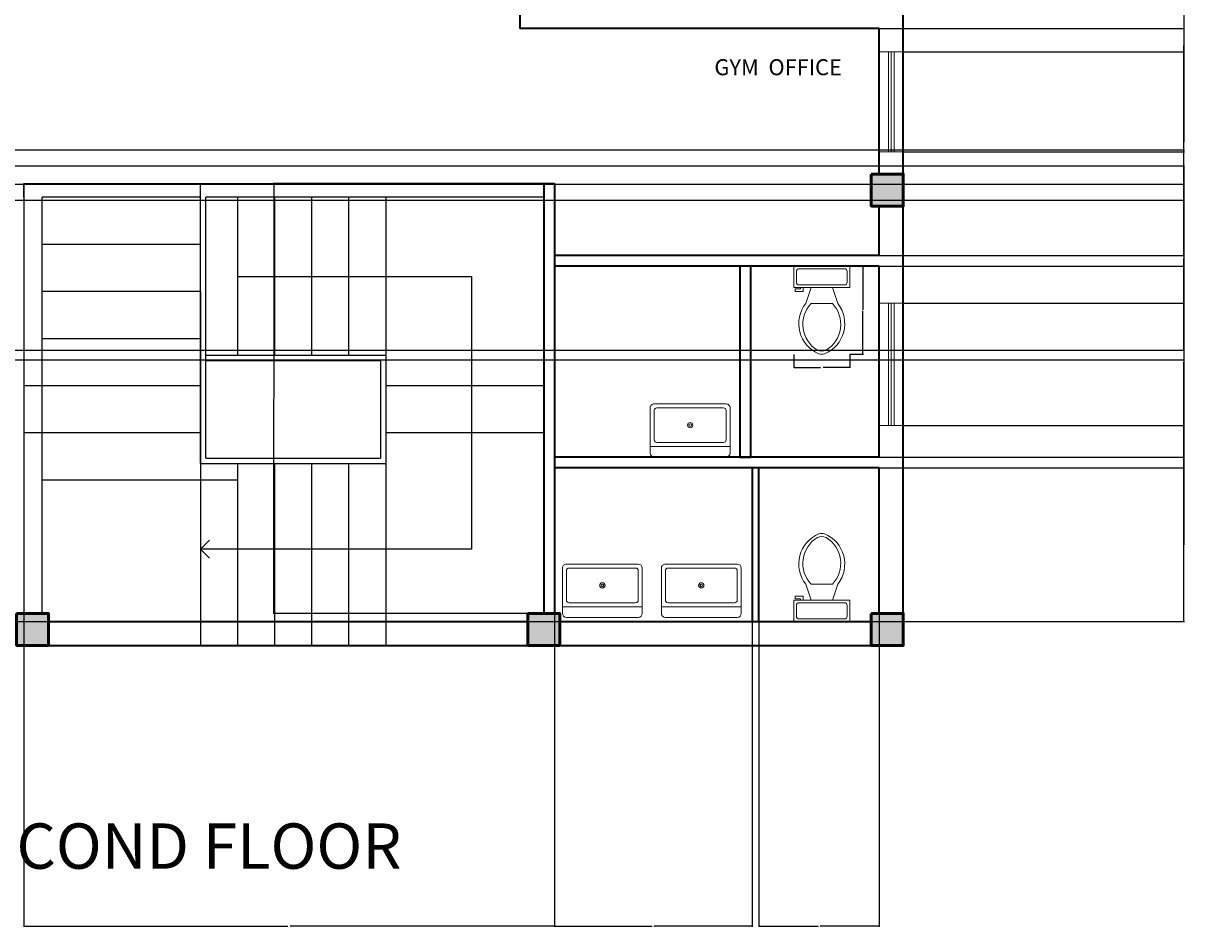
# Model space of a CAD drawing. Units: inches. Extents: x 369 to 4994, y 516 to 1297.
# Tile 8 of 9: x 2235 to 2672, y 516 to 855. Entities that reach past the tile are written whole.
import ezdxf

# ---------------------------------------------------------------- set-up
doc = ezdxf.new("R2010")
doc.units = ezdxf.units.IN
doc.header["$MEASUREMENT"] = 0
for name, color, linetype, lineweight in [('A-ANNO-DIMS', 2, 'Continuous', 18), ('A-ANNO-TEXT', 7, 'Continuous', 35), ('A-AREA-IDEN', 7, 'Continuous', 18), ('A-COLS', 7, 'Continuous', 50), ('A-FLOR-FIXT', 9, 'Continuous', 18), ('A-FLOR-STRS', 3, 'Continuous', 25), ('A-GLAZ', 4, 'Continuous', 18), ('A-WALL', 7, 'Continuous', 35)]:
    doc.layers.add(name, color=color, linetype=linetype, lineweight=lineweight)
doc.layers.add('A-COLS-PATT', color=18, linetype='Continuous', lineweight=13, true_color=0x000000)
doc.styles.get("Standard").update_dxf_attribs({"font": 'arial.ttf'})
doc.dimstyles.get("Standard").update_dxf_attribs({"dimtxt": 0.18, "dimasz": 0.18, "dimexe": 0.18, "dimexo": 0.0625, "dimgap": 0.09, "dimtad": 0, "dimtih": 1, "dimtoh": 1, "dimdec": 4, "dimzin": 0, "dimdsep": 46, "dimtxsty": 'Standard', "dimcen": 0.09, "dimadec": 0, "dimazin": 0, "dimtfac": 1, "dimtdec": 4, "dimtofl": 0, "dimtmove": 0, "dimatfit": 3, "dimfxl": 1, "dimtolj": 1, "dimtzin": 0, "dimarcsym": 0})

# ---------------------------------------------------------------- blocks, each defined once
blk = doc.blocks.new('Toilet - top')
for p, q in [((9.5, -6), (9.5, -2)), ((-10, -8.5), (-8, -8.5)), ((-10, -9.5), (-10, -8.5)), ((-8, -8.5), (-8, -8)), ((-7, -8), (-7, -9.5)), ((-4, -8), (-6, -14)), ((4, -8), (6, -14)), ((-7, -9.5), (-10, -9.5)), ((4, -14), (-4, -14))]:
    blk.add_line(p, q)
blk.add_lwpolyline([(10.5, -8), (10.5, 0), (-10.5, 0), (-10.5, -8)], close=True)
for points in [[(-9.5, -2), (-9.5, -6)], [(8.5, -1), (-8.5, -1)], [(-8.5, -7), (8.5, -7)]]:
    blk.add_lwpolyline(points)
for centre, radius, start, end in [((-8.62, -1.88), 0.884, 81.8699, 188.1301), ((8.62, -1.88), 0.884, 351.8699, 98.1301), ((-8.62, -6.12), 0.884, 171.8699, 278.1301), ((8.62, -6.12), 0.884, 261.8699, 8.1301), ((3.52, -21.58), 12.17, 141.4691, 247.9714), ((4.2, -21.82), 11.33, 136.3677, 238.9468), ((-3.52, -21.58), 12.17, 292.0284, 38.5307), ((-4.2, -21.82), 11.33, 301.053, 43.6321), ((0, -27.88), 4, 245.7318, 294.2682), ((0, -29), 4, 254.8605, 285.1395)]:
    blk.add_arc(centre, radius, start, end)
blk = doc.blocks.new('Sink-single - 30 in top')
blk.add_line((-15, -3.999996), (15, -3.999996))
for points in [[(-13.5, 0), (13.5, 0)], [(-15, -18.499996), (-15, -1.5)], [(15, -1.5), (15, -18.499996)], [(-13.5, -17.499996), (-13.5, -6.499996)], [(-12.5, -5.499996), (12.5, -5.499996)], [(13.5, -6.499996), (13.5, -17.499996)], [(13.5, -19.999996), (-13.5, -19.999996)], [(12.5, -18.499996), (-12.5, -18.499996)]]:
    blk.add_lwpolyline(points)
for radius in [1, 0.5]:
    blk.add_circle((0, -11.999996), radius)
for centre, radius, start, end in [((-13.5, -1.5), 1.5, 90, 180), ((13.5, -1.5), 1.5, 0, 90), ((-12.5, -6.499996), 1, 90, 180), ((12.5, -6.499996), 1, 0, 90), ((-13.5, -18.499996), 1.5, 180, 270), ((-12.5, -17.499996), 1, 180, 270), ((12.5, -17.499996), 1, 270, 0), ((13.5, -18.499996), 1.5, 270, 0)]:
    blk.add_arc(centre, radius, start, end)
blk = doc.blocks.new('*D25')
at = {"layer": 'A-ANNO-DIMS', "color": 0, "lineweight": -2, "transparency": 16777216}
for p, q in [((2545.87, 764.15), (2550.95, 764.15)), ((2550.77, 763.97), (2550.77, 747.81)), ((2550.77, 731.28), (2550.77, 747.44)), ((2545.87, 731.1), (2550.95, 731.1))]:
    blk.add_line(p, q, dxfattribs=at)
at = {"layer": 'A-ANNO-DIMS', "color": 0, "transparency": 16777216}
for points in [[(2550.74, 763.97), (2550.8, 763.97), (2550.77, 764.15)], [(2550.74, 731.28), (2550.8, 731.28), (2550.77, 731.1)]]:
    blk.add_solid(points, dxfattribs=at)
at = {"layer": 'Defpoints', "color": 0, "transparency": 16777216}
for p in [(2545.81, 764.15), (2550.77, 764.15), (2545.81, 731.1)]:
    blk.add_point(p, dxfattribs=at)
at = {"layer": 'A-ANNO-DIMS', "color": 0, "transparency": 16777216, "insert": (2550.77, 747.63), "char_height": 0.18, "attachment_point": 5}
blk.add_mtext('\\A1;WC 33 TYP.', dxfattribs=at)
blk = doc.blocks.new('*D26')
at = {"layer": 'A-ANNO-DIMS', "color": 0, "lineweight": -2, "transparency": 16777216}
for p, q in [((2524.81, 731.04), (2524.81, 725.97)), ((2545.81, 731.04), (2545.81, 725.97)), ((2524.99, 726.15), (2534.78, 726.15)), ((2545.63, 726.15), (2535.84, 726.15))]:
    blk.add_line(p, q, dxfattribs=at)
at = {"layer": 'A-ANNO-DIMS', "color": 0, "transparency": 16777216}
for points in [[(2524.99, 726.18), (2524.99, 726.12), (2524.81, 726.15)], [(2545.63, 726.18), (2545.63, 726.12), (2545.81, 726.15)]]:
    blk.add_solid(points, dxfattribs=at)
at = {"layer": 'Defpoints', "color": 0, "transparency": 16777216}
for p in [(2524.81, 731.1), (2545.81, 731.1), (2545.81, 726.15)]:
    blk.add_point(p, dxfattribs=at)
at = {"layer": 'A-ANNO-DIMS', "color": 0, "transparency": 16777216, "insert": (2535.31, 726.15), "char_height": 0.18, "attachment_point": 5}
blk.add_mtext('\\A1;21 TYP.', dxfattribs=at)
blk = doc.blocks.new('*D47')
at = {"layer": 'A-ANNO-DIMS', "color": 0, "lineweight": -2, "transparency": 16777216}
for p, q in [((1038.32, 879.79), (2671.51, 879.79)), ((2671.33, 879.61), (2671.33, 837.52)), ((2671.33, 795.07), (2671.33, 837.16)), ((1035.32, 794.89), (2671.51, 794.89))]:
    blk.add_line(p, q, dxfattribs=at)
at = {"layer": 'A-ANNO-DIMS', "color": 0, "transparency": 16777216}
for points in [[(2671.3, 879.61), (2671.36, 879.61), (2671.33, 879.79)], [(2671.3, 795.07), (2671.36, 795.07), (2671.33, 794.89)]]:
    blk.add_solid(points, dxfattribs=at)
at = {"layer": 'Defpoints', "color": 0, "transparency": 16777216}
for p in [(1038.26, 879.79), (2671.33, 879.79), (1035.26, 794.89)]:
    blk.add_point(p, dxfattribs=at)
at = {"layer": 'A-ANNO-DIMS', "color": 0, "transparency": 16777216, "insert": (2671.33, 837.34), "char_height": 0.18, "attachment_point": 5}
blk.add_mtext('\\A1;84.9', dxfattribs=at)
blk = doc.blocks.new('*D52')
at = {"layer": 'A-ANNO-DIMS', "color": 0, "lineweight": -2, "transparency": 16777216}
for p, q in [((942.32, 788.89), (2671.51, 788.89)), ((2671.33, 788.71), (2671.33, 710.02)), ((2671.33, 630.97), (2671.33, 709.66)), ((1035.32, 630.79), (2671.51, 630.79))]:
    blk.add_line(p, q, dxfattribs=at)
at = {"layer": 'A-ANNO-DIMS', "color": 0, "transparency": 16777216}
for points in [[(2671.3, 788.71), (2671.36, 788.71), (2671.33, 788.89)], [(2671.3, 630.97), (2671.36, 630.97), (2671.33, 630.79)]]:
    blk.add_solid(points, dxfattribs=at)
at = {"layer": 'Defpoints', "color": 0, "transparency": 16777216}
for p in [(942.26, 788.89), (2671.33, 788.89), (1035.26, 630.79)]:
    blk.add_point(p, dxfattribs=at)
at = {"layer": 'A-ANNO-DIMS', "color": 0, "transparency": 16777216, "insert": (2671.33, 709.84), "char_height": 0.18, "attachment_point": 5}
blk.add_mtext('\\A1;158.1', dxfattribs=at)
blk = doc.blocks.new('*D80')
at = {"layer": 'A-ANNO-DIMS', "color": 0, "lineweight": -2, "transparency": 16777216}
for p, q in [((1772.44, 886.6), (2671.51, 886.6)), ((2671.33, 886.42), (2671.33, 847.38)), ((2671.33, 807.97), (2671.33, 847.01)), ((1772.44, 807.79), (2671.51, 807.79))]:
    blk.add_line(p, q, dxfattribs=at)
at = {"layer": 'A-ANNO-DIMS', "color": 0, "transparency": 16777216}
for points in [[(2671.3, 886.42), (2671.36, 886.42), (2671.33, 886.6)], [(2671.3, 807.97), (2671.36, 807.97), (2671.33, 807.79)]]:
    blk.add_solid(points, dxfattribs=at)
at = {"layer": 'Defpoints', "color": 0, "transparency": 16777216}
for p in [(1772.37, 886.6), (2671.33, 886.6), (1772.37, 807.79)]:
    blk.add_point(p, dxfattribs=at)
at = {"layer": 'A-ANNO-DIMS', "color": 0, "transparency": 16777216, "insert": (2671.33, 847.19), "char_height": 0.18, "attachment_point": 5}
blk.add_mtext('\\A1;78.81', dxfattribs=at)
blk = doc.blocks.new('*D85')
at = {"layer": 'A-ANNO-DIMS', "color": 0, "lineweight": -2, "transparency": 16777216}
for p, q in [((1772.44, 801.79), (2671.51, 801.79)), ((2671.33, 801.61), (2671.33, 767.36)), ((2671.33, 732.75), (2671.33, 767)), ((1772.44, 732.57), (2671.51, 732.57))]:
    blk.add_line(p, q, dxfattribs=at)
at = {"layer": 'A-ANNO-DIMS', "color": 0, "transparency": 16777216}
for points in [[(2671.3, 801.61), (2671.36, 801.61), (2671.33, 801.79)], [(2671.3, 732.75), (2671.36, 732.75), (2671.33, 732.57)]]:
    blk.add_solid(points, dxfattribs=at)
at = {"layer": 'Defpoints', "color": 0, "transparency": 16777216}
for p in [(1772.37, 801.79), (2671.33, 801.79), (1772.37, 732.57)]:
    blk.add_point(p, dxfattribs=at)
at = {"layer": 'A-ANNO-DIMS', "color": 0, "transparency": 16777216, "insert": (2671.33, 767.18), "char_height": 0.18, "attachment_point": 5}
blk.add_mtext('\\A1;69.22', dxfattribs=at)
blk = doc.blocks.new('*D86')
at = {"layer": 'A-ANNO-DIMS', "color": 0, "lineweight": -2, "transparency": 16777216}
for p, q in [((1772.44, 728.97), (2671.51, 728.97)), ((2671.33, 728.79), (2671.33, 680.06)), ((2671.33, 630.97), (2671.33, 679.7)), ((1769.44, 630.79), (2671.51, 630.79))]:
    blk.add_line(p, q, dxfattribs=at)
at = {"layer": 'A-ANNO-DIMS', "color": 0, "transparency": 16777216}
for points in [[(2671.3, 728.79), (2671.36, 728.79), (2671.33, 728.97)], [(2671.3, 630.97), (2671.36, 630.97), (2671.33, 630.79)]]:
    blk.add_solid(points, dxfattribs=at)
at = {"layer": 'Defpoints', "color": 0, "transparency": 16777216}
for p in [(1772.37, 728.97), (2671.33, 728.97), (1769.37, 630.79)]:
    blk.add_point(p, dxfattribs=at)
at = {"layer": 'A-ANNO-DIMS', "color": 0, "transparency": 16777216, "insert": (2671.33, 679.88), "char_height": 0.18, "attachment_point": 5}
blk.add_mtext('\\A1;98.18', dxfattribs=at)
blk = doc.blocks.new('*D105')
at = {"layer": 'A-ANNO-DIMS', "color": 0, "lineweight": -2, "transparency": 16777216}
for p, q in [((2556.99, 853.34), (2671.51, 853.34)), ((2671.33, 853.16), (2671.33, 810.93)), ((2671.33, 768.33), (2671.33, 810.56)), ((2556.99, 768.15), (2671.51, 768.15))]:
    blk.add_line(p, q, dxfattribs=at)
at = {"layer": 'A-ANNO-DIMS', "color": 0, "transparency": 16777216}
for points in [[(2671.3, 853.16), (2671.36, 853.16), (2671.33, 853.34)], [(2671.3, 768.33), (2671.36, 768.33), (2671.33, 768.15)]]:
    blk.add_solid(points, dxfattribs=at)
at = {"layer": 'Defpoints', "color": 0, "transparency": 16777216}
for p in [(2556.93, 853.34), (2671.33, 853.34), (2556.93, 768.15)]:
    blk.add_point(p, dxfattribs=at)
at = {"layer": 'A-ANNO-DIMS', "color": 0, "transparency": 16777216, "insert": (2671.33, 810.75), "char_height": 0.18, "attachment_point": 5}
blk.add_mtext('\\A1;85.19', dxfattribs=at)
blk = doc.blocks.new('*D106')
at = {"layer": 'A-ANNO-DIMS', "color": 0, "lineweight": -2, "transparency": 16777216}
for p, q in [((2556.99, 764.15), (2671.51, 764.15)), ((2671.33, 763.97), (2671.33, 728.5)), ((2671.33, 692.66), (2671.33, 728.13)), ((2556.99, 692.48), (2671.51, 692.48))]:
    blk.add_line(p, q, dxfattribs=at)
at = {"layer": 'A-ANNO-DIMS', "color": 0, "transparency": 16777216}
for points in [[(2671.3, 763.97), (2671.36, 763.97), (2671.33, 764.15)], [(2671.3, 692.66), (2671.36, 692.66), (2671.33, 692.48)]]:
    blk.add_solid(points, dxfattribs=at)
at = {"layer": 'Defpoints', "color": 0, "transparency": 16777216}
for p in [(2556.93, 764.15), (2671.33, 764.15), (2556.93, 692.48)]:
    blk.add_point(p, dxfattribs=at)
at = {"layer": 'A-ANNO-DIMS', "color": 0, "transparency": 16777216, "insert": (2671.33, 728.32), "char_height": 0.18, "attachment_point": 5}
blk.add_mtext('\\A1;71.67', dxfattribs=at)
blk = doc.blocks.new('*D107')
at = {"layer": 'A-ANNO-DIMS', "color": 0, "lineweight": -2, "transparency": 16777216}
for p, q in [((2556.99, 688.48), (2671.51, 688.48)), ((2671.33, 688.3), (2671.33, 659.82)), ((2671.33, 630.97), (2671.33, 659.45)), ((2553.99, 630.79), (2671.51, 630.79))]:
    blk.add_line(p, q, dxfattribs=at)
at = {"layer": 'A-ANNO-DIMS', "color": 0, "transparency": 16777216}
for points in [[(2671.3, 688.3), (2671.36, 688.3), (2671.33, 688.48)], [(2671.3, 630.97), (2671.36, 630.97), (2671.33, 630.79)]]:
    blk.add_solid(points, dxfattribs=at)
at = {"layer": 'Defpoints', "color": 0, "transparency": 16777216}
for p in [(2556.93, 688.48), (2671.33, 688.48), (2553.93, 630.79)]:
    blk.add_point(p, dxfattribs=at)
at = {"layer": 'A-ANNO-DIMS', "color": 0, "transparency": 16777216, "insert": (2671.33, 659.64), "char_height": 0.18, "attachment_point": 5}
blk.add_mtext('\\A1;57.69', dxfattribs=at)
blk = doc.blocks.new('*D109')
at = {"layer": 'A-ANNO-DIMS', "color": 0, "lineweight": -2, "transparency": 16777216}
for p, q in [((2235.65, 795.12), (2235.65, 516.21)), ((2434.93, 795.12), (2434.93, 516.21)), ((2235.83, 516.39), (2334.83, 516.39)), ((2434.75, 516.39), (2335.74, 516.39))]:
    blk.add_line(p, q, dxfattribs=at)
at = {"layer": 'A-ANNO-DIMS', "color": 0, "transparency": 16777216}
for points in [[(2235.83, 516.42), (2235.83, 516.36), (2235.65, 516.39)], [(2434.75, 516.42), (2434.75, 516.36), (2434.93, 516.39)]]:
    blk.add_solid(points, dxfattribs=at)
at = {"layer": 'Defpoints', "color": 0, "transparency": 16777216}
for p in [(2235.65, 795.19), (2434.93, 795.19), (2434.93, 516.39)]:
    blk.add_point(p, dxfattribs=at)
at = {"layer": 'A-ANNO-DIMS', "color": 0, "transparency": 16777216, "insert": (2335.29, 516.39), "char_height": 0.18, "attachment_point": 5}
blk.add_mtext('\\A1;199.27', dxfattribs=at)
blk = doc.blocks.new('*D110')
at = {"layer": 'A-ANNO-DIMS', "color": 0, "lineweight": -2, "transparency": 16777216}
for p, q in [((2434.93, 688.42), (2434.93, 516.21)), ((2509.12, 688.42), (2509.12, 516.21)), ((2435.11, 516.39), (2471.63, 516.39)), ((2508.94, 516.39), (2472.42, 516.39))]:
    blk.add_line(p, q, dxfattribs=at)
at = {"layer": 'A-ANNO-DIMS', "color": 0, "transparency": 16777216}
for points in [[(2435.11, 516.42), (2435.11, 516.36), (2434.93, 516.39)], [(2508.94, 516.42), (2508.94, 516.36), (2509.12, 516.39)]]:
    blk.add_solid(points, dxfattribs=at)
at = {"layer": 'Defpoints', "color": 0, "transparency": 16777216}
for p in [(2434.93, 688.48), (2509.12, 688.48), (2509.12, 516.39)]:
    blk.add_point(p, dxfattribs=at)
at = {"layer": 'A-ANNO-DIMS', "color": 0, "transparency": 16777216, "insert": (2472.02, 516.39), "char_height": 0.18, "attachment_point": 5}
blk.add_mtext('\\A1;74.19', dxfattribs=at)
blk = doc.blocks.new('*D111')
at = {"layer": 'A-ANNO-DIMS', "color": 0, "lineweight": -2, "transparency": 16777216}
for p, q in [((2511.66, 688.42), (2511.66, 516.21)), ((2556.93, 688.42), (2556.93, 516.21)), ((2511.84, 516.39), (2533.9, 516.39)), ((2556.75, 516.39), (2534.69, 516.39))]:
    blk.add_line(p, q, dxfattribs=at)
at = {"layer": 'A-ANNO-DIMS', "color": 0, "transparency": 16777216}
for points in [[(2511.84, 516.42), (2511.84, 516.36), (2511.66, 516.39)], [(2556.75, 516.42), (2556.75, 516.36), (2556.93, 516.39)]]:
    blk.add_solid(points, dxfattribs=at)
at = {"layer": 'Defpoints', "color": 0, "transparency": 16777216}
for p in [(2511.66, 688.48), (2556.93, 688.48), (2556.93, 516.39)]:
    blk.add_point(p, dxfattribs=at)
at = {"layer": 'A-ANNO-DIMS', "color": 0, "transparency": 16777216, "insert": (2534.29, 516.39), "char_height": 0.18, "attachment_point": 5}
blk.add_mtext('\\A1;45.27', dxfattribs=at)
blk = doc.blocks.new('*D118')
at = {"layer": 'A-ANNO-DIMS', "color": 0, "lineweight": -2, "transparency": 16777216}
for p, q in [((2565.99, 844.57), (2671.51, 844.57)), ((2671.33, 844.39), (2671.33, 826.03)), ((2671.33, 807.3), (2671.33, 825.66)), ((2565.99, 807.12), (2671.51, 807.12))]:
    blk.add_line(p, q, dxfattribs=at)
at = {"layer": 'A-ANNO-DIMS', "color": 0, "transparency": 16777216}
for points in [[(2671.3, 844.39), (2671.36, 844.39), (2671.33, 844.57)], [(2671.3, 807.3), (2671.36, 807.3), (2671.33, 807.12)]]:
    blk.add_solid(points, dxfattribs=at)
at = {"layer": 'Defpoints', "color": 0, "transparency": 16777216}
for p in [(2565.93, 844.57), (2565.93, 807.12), (2671.33, 807.12)]:
    blk.add_point(p, dxfattribs=at)
at = {"layer": 'A-ANNO-DIMS', "color": 0, "transparency": 16777216, "insert": (2671.33, 825.84), "char_height": 0.18, "attachment_point": 5}
blk.add_mtext('\\A1;37.45', dxfattribs=at)
blk = doc.blocks.new('*D119')
at = {"layer": 'A-ANNO-DIMS', "color": 0, "lineweight": -2, "transparency": 16777216}
for p, q in [((2565.99, 750.32), (2671.51, 750.32)), ((2671.33, 750.14), (2671.33, 727.55)), ((2671.33, 704.59), (2671.33, 727.18)), ((2565.99, 704.41), (2671.51, 704.41))]:
    blk.add_line(p, q, dxfattribs=at)
at = {"layer": 'A-ANNO-DIMS', "color": 0, "transparency": 16777216}
for points in [[(2671.3, 750.14), (2671.36, 750.14), (2671.33, 750.32)], [(2671.3, 704.59), (2671.36, 704.59), (2671.33, 704.41)]]:
    blk.add_solid(points, dxfattribs=at)
at = {"layer": 'Defpoints', "color": 0, "transparency": 16777216}
for p in [(2565.93, 750.32), (2565.93, 704.41), (2671.33, 704.41)]:
    blk.add_point(p, dxfattribs=at)
at = {"layer": 'A-ANNO-DIMS', "color": 0, "transparency": 16777216, "insert": (2671.33, 727.36), "char_height": 0.18, "attachment_point": 5}
blk.add_mtext('\\A1;45.91', dxfattribs=at)
blk = doc.blocks.new('*D121')
at = {"layer": 'A-ANNO-DIMS', "color": 0, "lineweight": -2, "transparency": 16777216}
for p, q in [((2434.86, 795.19), (2329.35, 795.19)), ((2329.53, 795.01), (2329.53, 714.67)), ((2329.53, 633.97), (2329.53, 714.31)), ((2434.86, 633.79), (2329.35, 633.79))]:
    blk.add_line(p, q, dxfattribs=at)
at = {"layer": 'A-ANNO-DIMS', "color": 0, "transparency": 16777216}
for points in [[(2329.5, 795.01), (2329.56, 795.01), (2329.53, 795.19)], [(2329.5, 633.97), (2329.56, 633.97), (2329.53, 633.79)]]:
    blk.add_solid(points, dxfattribs=at)
at = {"layer": 'Defpoints', "color": 0, "transparency": 16777216}
for p in [(2329.53, 795.19), (2434.93, 795.19), (2434.93, 633.79)]:
    blk.add_point(p, dxfattribs=at)
at = {"layer": 'A-ANNO-DIMS', "color": 0, "transparency": 16777216, "insert": (2329.53, 714.49), "char_height": 0.18, "attachment_point": 5}
blk.add_mtext('\\A1;161.4', dxfattribs=at)

msp = doc.modelspace()

# ---------------------------------------------------------------- hatches: boundary and pattern name
at = {"layer": 'A-COLS-PATT'}
h = msp.add_hatch(color=256, dxfattribs=at)
h.dxf.hatch_style = 1
h.paths.add_polyline_path([(540.2581, 633.7894), (528.2581, 633.7894), (528.2581, 621.7894), (540.2581, 621.7894)])
h.paths.add_polyline_path([(726.2581, 633.7894), (714.2581, 633.7894), (714.2581, 621.7894), (726.2581, 621.7894)])
h.paths.add_polyline_path([(918.2581, 633.7894), (906.2581, 633.7894), (906.2581, 621.7894), (918.2581, 621.7894)])
h.paths.add_polyline_path([(1047.2581, 633.7894), (1035.2581, 633.7894), (1035.2581, 621.7894), (1047.2581, 621.7894)])
h.paths.add_polyline_path([(1047.2581, 798.6977), (1035.2581, 798.6977), (1035.2581, 786.6977), (1047.2581, 786.6977)])
h.paths.add_polyline_path([(918.2581, 795.7894), (906.2581, 795.7894), (906.2581, 783.7894), (918.2581, 783.7894)])
h.paths.add_polyline_path([(726.2581, 795.7894), (714.2581, 795.7894), (714.2581, 783.7894), (726.2581, 783.7894)])
h.paths.add_polyline_path([(1047.2581, 1038.7894), (1035.2581, 1038.7894), (1035.2581, 1026.7894), (1047.2581, 1026.7894)])
h.paths.add_polyline_path([(855.044, 1038.7894), (843.044, 1038.7894), (843.044, 1026.7894), (855.044, 1026.7894)])
h.paths.add_polyline_path([(728.5536, 1038.7894), (716.5536, 1038.7894), (716.5536, 1026.7894), (728.5536, 1026.7894)])
h.paths.add_polyline_path([(543.2581, 1038.7894), (531.2581, 1038.7894), (531.2581, 1026.7894), (543.2581, 1026.7894)])
h.paths.add_polyline_path([(543.2581, 792.9013), (531.2581, 792.9013), (531.2581, 780.9013), (543.2581, 780.9013), (543.2581, 783.7894)])
h.paths.add_polyline_path([(1274.3738, 633.7894), (1262.3738, 633.7894), (1262.3738, 621.7894), (1274.3738, 621.7894)])
h.paths.add_polyline_path([(1460.3738, 633.7894), (1448.3738, 633.7894), (1448.3738, 621.7894), (1460.3738, 621.7894)])
h.paths.add_polyline_path([(1652.3738, 633.7894), (1640.3738, 633.7894), (1640.3738, 621.7894), (1652.3738, 621.7894)])
h.paths.add_polyline_path([(1781.3738, 633.7894), (1769.3738, 633.7894), (1769.3738, 621.7894), (1781.3738, 621.7894)])
h.paths.add_polyline_path([(1781.3738, 1038.7894), (1769.3738, 1038.7894), (1769.3738, 1026.7894), (1781.3738, 1026.7894)])
h.paths.add_polyline_path([(1625.484, 1038.7894), (1613.484, 1038.7894), (1613.484, 1026.7894), (1615.6962, 1026.7894), (1625.484, 1026.7894)])
h.paths.add_polyline_path([(1462.6692, 1038.7894), (1450.6692, 1038.7894), (1450.6692, 1026.7894), (1462.6692, 1026.7894)])
h.paths.add_polyline_path([(1277.3738, 1038.7894), (1265.3738, 1038.7894), (1265.3738, 1026.7894), (1277.3738, 1026.7894)])
h.paths.add_polyline_path([(1460.3738, 807.7894), (1448.3738, 807.7894), (1448.3738, 795.7894), (1460.3738, 795.7894)])
h.paths.add_polyline_path([(1652.3738, 807.7894), (1640.3738, 807.7894), (1640.3738, 795.7894), (1652.3738, 795.7894)])
h.paths.add_polyline_path([(2244.9265, 633.7894), (2232.9265, 633.7894), (2232.9265, 621.7894), (2244.9265, 621.7894)])
h.paths.add_polyline_path([(2058.9265, 633.7894), (2046.9265, 633.7894), (2046.9265, 621.7894), (2058.9265, 621.7894)])
h.paths.add_polyline_path([(2436.9265, 633.7894), (2424.9265, 633.7894), (2424.9265, 621.7894), (2436.9265, 621.7894)])
h.paths.add_polyline_path([(2565.9265, 633.7894), (2553.9265, 633.7894), (2553.9265, 621.7894), (2565.9265, 621.7894)])
h.paths.add_polyline_path([(2565.9265, 798.6977), (2553.9265, 798.6977), (2553.9265, 786.6977), (2565.9265, 786.6977)])
h.paths.add_polyline_path([(2565.9265, 1038.7894), (2553.9265, 1038.7894), (2553.9265, 1026.7894), (2565.9265, 1026.7894)])
h.paths.add_polyline_path([(2436.9265, 1038.7894), (2424.9265, 1038.7894), (2424.9265, 1026.7894), (2436.9265, 1026.7894)])
h.paths.add_polyline_path([(2247.222, 1038.7894), (2235.222, 1038.7894), (2235.222, 1026.7894), (2247.222, 1026.7894)])
h.paths.add_polyline_path([(2061.9265, 1038.7894), (2049.9265, 1038.7894), (2049.9265, 1026.7894), (2061.9265, 1026.7894)])

# ---------------------------------------------------------------- linework, layer by layer
at = {"layer": 'A-COLS'}
for points in [[(2553.9265, 798.6977), (2565.9265, 798.6977), (2565.9265, 786.6977), (2553.9265, 786.6977)], [(2232.9265, 633.7894), (2244.9265, 633.7894), (2244.9265, 621.7894), (2232.9265, 621.7894)], [(2424.9265, 633.7894), (2436.9265, 633.7894), (2436.9265, 621.7894), (2424.9265, 621.7894)], [(2553.9265, 633.7894), (2565.9265, 633.7894), (2565.9265, 621.7894), (2553.9265, 621.7894)]]:
    msp.add_lwpolyline(points, close=True, dxfattribs=at)
at = {"layer": 'A-FLOR-STRS'}
for p, q in [((2235.6525, 795.1866), (2235.6525, 633.7894)), ((2301.9505, 690.1533), (2301.9505, 795.1866)), ((2430.9265, 795.1866), (2434.9265, 795.1866)), ((2242.5867, 633.7894), (2242.5867, 790.0048)), ((2303.9505, 692.1533), (2303.9505, 790.0048)), ((2315.873, 790.0048), (2315.873, 730.6409)), ((2329.7954, 790.0048), (2329.7954, 730.6409)), ((2343.7178, 790.0048), (2343.7178, 730.6409)), ((2357.6402, 790.0048), (2357.6402, 730.6409)), ((2371.5626, 790.0048), (2371.5626, 621.7894)), ((2371.5626, 790.0048), (2371.5626, 621.7894)), ((2315.873, 760.3228), (2403.7562, 760.3228)), ((2403.7562, 760.3228), (2403.7562, 657.9608)), ((2301.9505, 754.6236), (2301.9505, 621.7894)), ((2369.5626, 728.6409), (2369.5626, 692.1533)), ((2371.5626, 730.6409), (2371.5626, 690.1533)), ((2301.9505, 690.1533), (2371.5626, 690.1533)), ((2303.9505, 692.1533), (2369.5626, 692.1533)), ((2315.873, 690.1533), (2315.873, 621.7894)), ((2329.7954, 690.1533), (2329.7954, 621.7894)), ((2343.7178, 690.1533), (2343.7178, 621.7894)), ((2357.6402, 690.1533), (2357.6402, 621.7894)), ((2301.9505, 657.9608), (2305.3296, 661.3398)), ((2403.7562, 657.9608), (2301.9505, 657.9608)), ((2301.9505, 657.9608), (2305.3296, 654.5817)), ((2235.6525, 633.7894), (2242.5867, 633.7894)), ((2303.9505, 630.7894), (2369.5626, 630.7894))]:
    msp.add_line(p, q, dxfattribs=at)
for points in [[(2235.6525, 790.0048), (2235.6525, 795.1866), (2430.9265, 795.1866)], [(2301.9505, 790.0048), (2242.5867, 790.0048)], [(2430.9265, 790.0048), (2303.9505, 790.0048)], [(2301.9505, 772.3142), (2242.5867, 772.3142)], [(2301.9505, 754.6236), (2242.5867, 754.6236)], [(2301.9505, 736.933), (2242.5867, 736.933)], [(2371.5626, 730.6409), (2303.9505, 730.6409)], [(2369.5626, 728.6409), (2303.9505, 728.6409)], [(2301.9505, 719.2424), (2235.6525, 719.2424)], [(2430.9265, 719.2424), (2371.5626, 719.2424)], [(2301.9505, 701.5518), (2235.6525, 701.5518)], [(2430.9265, 701.5518), (2371.5626, 701.5518)], [(2315.873, 683.8612), (2242.5867, 683.8612)], [(2301.9505, 630.7894), (2244.9265, 630.7894)]]:
    msp.add_lwpolyline(points, dxfattribs=at)
at = {"layer": 'A-GLAZ'}
for p, q in [((2560.3504, 807.1195), (2560.3504, 844.5673)), ((2561.4265, 807.1195), (2561.4265, 844.5673)), ((2562.5026, 807.1195), (2562.5026, 844.5673)), ((2560.3504, 704.4093), (2560.3504, 750.3191)), ((2561.4265, 704.4093), (2561.4265, 750.3191)), ((2562.5026, 704.4093), (2562.5026, 750.3191))]:
    msp.add_line(p, q, dxfattribs=at)
for points in [[(2556.9265, 807.1195), (2565.9265, 807.1195), (2565.9265, 844.5673), (2556.9265, 844.5673)], [(2556.9265, 704.4093), (2565.9265, 704.4093), (2565.9265, 750.3191), (2556.9265, 750.3191)]]:
    msp.add_lwpolyline(points, close=True, dxfattribs=at)
at = {"layer": 'A-WALL'}
for p, q in [((2565.9265, 621.7894), (2565.9265, 1029.7894)), ((2421.9265, 908.8078), (2421.9265, 853.3402)), ((2430.9265, 853.3402), (2421.9265, 853.3402)), ((2556.9265, 853.3402), (2430.9265, 853.3402)), ((2556.9265, 798.6977), (2556.9265, 853.3402)), ((2556.9265, 798.6977), (2556.9265, 853.3402)), ((2430.9265, 795.1866), (2430.9265, 768.15)), ((2430.9265, 795.1866), (2430.9265, 633.7894)), ((2434.9265, 795.1866), (2434.9265, 688.4833)), ((2556.9265, 771.7894), (2556.9265, 786.6977)), ((2556.9265, 768.15), (2556.9265, 786.6977)), ((2556.9265, 768.15), (2434.9265, 768.15)), ((2434.9265, 768.15), (2434.9265, 692.4833)), ((2556.9265, 764.15), (2434.9265, 764.15)), ((2556.9265, 692.4833), (2556.9265, 764.15)), ((2430.9265, 692.4833), (2430.9265, 633.7894)), ((2556.9265, 692.4833), (2434.9265, 692.4833)), ((2556.9265, 688.4833), (2434.9265, 688.4833)), ((2434.9265, 688.4833), (2434.9265, 633.7894)), ((2556.9265, 633.7894), (2556.9265, 688.4833)), ((2244.9265, 630.7894), (2424.9265, 630.7894)), ((2436.9265, 630.7894), (2466.1551, 630.7894)), ((2436.9265, 630.7894), (2553.9265, 630.7894)), ((2244.9265, 621.7894), (2436.9265, 621.7894)), ((2436.9265, 621.7894), (2565.9265, 621.7894))]:
    msp.add_line(p, q, dxfattribs=at)
for points in [[(2504.5834, 692.4833), (2508.6491, 692.4833), (2508.6491, 764.15), (2504.5834, 764.15)], [(2509.1182, 630.7894), (2511.6597, 630.7894), (2511.6597, 688.4833), (2509.1182, 688.4833)]]:
    msp.add_lwpolyline(points, close=True, dxfattribs=at)

# ---------------------------------------------------------------- block references
at = {"layer": 'A-FLOR-FIXT'}
msp.add_blockref('Toilet - top', (2535.3093, 764.15), dxfattribs=at)
at = {"layer": 'A-FLOR-FIXT', "rotation": 180}
for p in [(2485.9052, 692.4833), (2452.9154, 632.3406), (2490.0727, 632.3406)]:
    msp.add_blockref('Sink-single - 30 in top', p, dxfattribs=at)
at = {"layer": 'A-FLOR-FIXT', "xscale": -1, "rotation": 180}
msp.add_blockref('Toilet - top', (2535.3093, 630.7894), dxfattribs=at)

# ---------------------------------------------------------------- texts
at = {"layer": 'A-ANNO-TEXT'}
msp.add_text('SECOND FLOOR', height=17.017766, dxfattribs=at).set_placement((2205.3764, 537.9843))
at = {"layer": 'A-AREA-IDEN'}
msp.add_text(' GYM  OFFICE', height=6, dxfattribs=at).set_placement((2493.1647, 835.8291))

# ---------------------------------------------------------------- dimensions: what is measured, and where the dimension line sits
at = {"layer": 'A-ANNO-DIMS'}
for base, p1, p2, angle, override, picture, middle in [((2671.3265, 886.5988), (1772.3738, 807.7894), (1772.3738, 886.5988), 90, {"dimdec": 2, "dimlfac": 1, "dimrnd": 0, "dimzin": 0, "dimdsep": 46, "dimlunit": 2}, '*D80', (2671.3265, 847.1941)), ((2671.3265, 879.7894), (1035.2581, 794.8925), (1038.2581, 879.7894), 90, {"dimdec": 1, "dimlfac": 1, "dimrnd": 0, "dimzin": 0, "dimdsep": 46, "dimlunit": 2}, '*D47', (2671.3265, 837.3409)), ((2671.3265, 853.3402), (2556.9265, 768.15), (2556.9265, 853.3402), 90, {"dimdec": 2, "dimlfac": 1, "dimrnd": 0, "dimzin": 0, "dimdsep": 46, "dimlunit": 2}, '*D105', (2671.3265, 810.7451)), ((2671.3265, 807.1195), (2565.9265, 844.5673), (2565.9265, 807.1195), 270, {"dimdec": 2, "dimlfac": 1, "dimrnd": 0, "dimzin": 0, "dimdsep": 46, "dimlunit": 2}, '*D118', (2671.3265, 825.8434)), ((2671.3265, 801.7894), (1772.3738, 732.5675), (1772.3738, 801.7894), 90, {"dimdec": 2, "dimlfac": 1, "dimrnd": 0, "dimzin": 0, "dimdsep": 46, "dimlunit": 2}, '*D85', (2671.3265, 767.1784)), ((2329.5265, 795.1866), (2434.9265, 633.7894), (2434.9265, 795.1866), 90, {"dimdec": 1, "dimlfac": 1, "dimrnd": 0, "dimzin": 0, "dimdsep": 46, "dimlunit": 2}, '*D121', (2329.5265, 714.488)), ((2671.3265, 788.8925), (1035.2581, 630.7894), (942.2581, 788.8925), 90, {"dimdec": 1, "dimlfac": 1, "dimrnd": 0, "dimzin": 0, "dimdsep": 46, "dimlunit": 2}, '*D52', (2671.3265, 709.8409)), ((2671.3265, 764.15), (2556.9265, 692.4833), (2556.9265, 764.15), 90, {"dimdec": 2, "dimlfac": 1, "dimrnd": 0, "dimzin": 0, "dimdsep": 46, "dimlunit": 2}, '*D106', (2671.3265, 728.3167)), ((2671.3265, 704.4093), (2565.9265, 750.3191), (2565.9265, 704.4093), 270, {"dimdec": 2, "dimlfac": 1, "dimrnd": 0, "dimzin": 0, "dimdsep": 46, "dimlunit": 2}, '*D119', (2671.3265, 727.3642)), ((2671.3265, 728.9712), (1769.3738, 630.7894), (1772.3738, 728.9712), 90, {"dimdec": 2, "dimlfac": 1, "dimrnd": 0, "dimzin": 0, "dimdsep": 46, "dimlunit": 2}, '*D86', (2671.3265, 679.8803)), ((2671.3265, 688.4833), (2553.9265, 630.7894), (2556.9265, 688.4833), 90, {"dimdec": 2, "dimlfac": 1, "dimrnd": 0, "dimzin": 0, "dimdsep": 46, "dimlunit": 2}, '*D107', (2671.3265, 659.6364))]:
    dim = msp.add_linear_dim(base=base, p1=p1, p2=p2, angle=angle, dimstyle='Standard', override=override, dxfattribs=at)
    dim.commit()
    dim.dimension.update_dxf_attribs({"geometry": picture, "text_midpoint": middle})
for base, p1, p2, picture, middle in [((2434.9265, 516.3894), (2235.6525, 795.1866), (2434.9265, 795.1866), '*D109', (2335.2895, 516.3894)), ((2509.1182, 516.3894), (2434.9265, 688.4833), (2509.1182, 688.4833), '*D110', (2472.0223, 516.3894)), ((2556.9265, 516.3894), (2511.6597, 688.4833), (2556.9265, 688.4833), '*D111', (2534.2931, 516.3894))]:
    dim = msp.add_linear_dim(base=base, p1=p1, p2=p2, dimstyle='Standard', override={"dimdec": 2, "dimlfac": 1, "dimrnd": 0, "dimzin": 0, "dimdsep": 46, "dimlunit": 2}, dxfattribs=at)
    dim.commit()
    dim.dimension.update_dxf_attribs({"geometry": picture, "text_midpoint": middle})
dim = msp.add_linear_dim(base=(2550.7662, 764.15), p1=(2545.8093, 731.1038), p2=(2545.8093, 764.15), angle=90, text='WC <> TYP.', dimstyle='Standard', override={"dimdec": 0, "dimlfac": 1, "dimrnd": 0, "dimzin": 0, "dimdsep": 46, "dimlunit": 2}, dxfattribs=at)
dim.commit()
dim.dimension.update_dxf_attribs({"geometry": '*D25', "text_midpoint": (2550.7662, 747.6269)})
dim = msp.add_linear_dim(base=(2545.8093, 726.1469), p1=(2524.8093, 731.1038), p2=(2545.8093, 731.1038), text='<> TYP.', dimstyle='Standard', override={"dimdec": 0, "dimlfac": 1, "dimrnd": 0, "dimzin": 0, "dimdsep": 46, "dimlunit": 2}, dxfattribs=at)
dim.commit()
dim.dimension.update_dxf_attribs({"geometry": '*D26', "text_midpoint": (2535.3093, 726.1469)})

doc.saveas('drawing.dxf')
